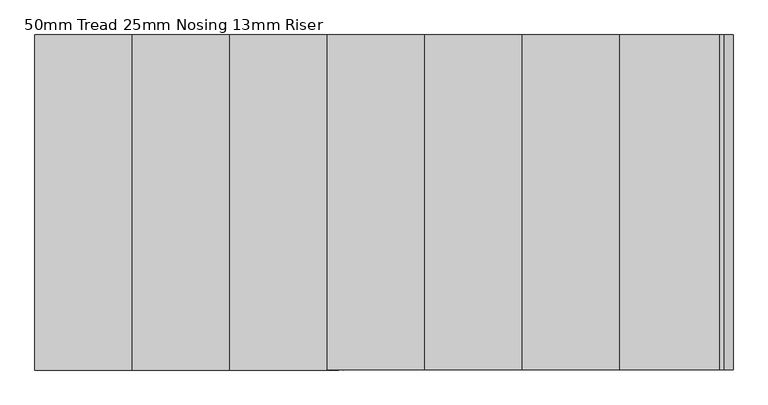
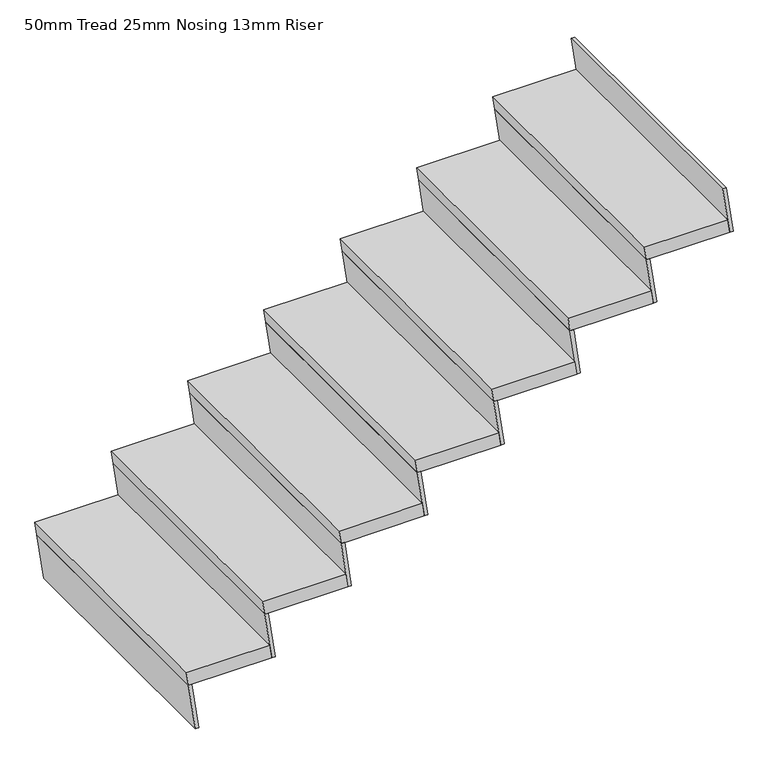
"""IFC4 building model written with IfcOpenShell, lengths in millimetres: stair flight geometry, 50mm Tread 25mm Nosing 13mm Riser."""

from ifc_helpers import new_model, si_unit, frame, origin, place, context, project, spatial, polyline, outline, extrude, source, transform, mapped, element, save


def stair_flight_50mm_tread_25mm_nosing_13mm_riser_6fe2c66d(model_context):
    return source(origin(), model_context, "Body", "SweptSolid", [
        extrude(outline(polyline([(1217.3913043, -932.4697153), (1217.3913043, -1232.4697153), (1167.3913043, -1225.2822153), (1167.3913043, -925.2822153), (1217.3913043, -932.4697153)])), frame((0.0, 1980.9593033, 0.0), z_axis=(0.0, 1.0, 0.0), x_axis=(0.0, 0.0, 1.0)), (0.0, 0.0, 1.0), 945.271643),
        extrude(outline(polyline([(1167.3913043, -1225.2822153), (993.4782609, -1200.2822153), (993.4782609, -1187.6537253), (1167.3913043, -1212.6537253), (1167.3913043, -1225.2822153)])), frame((0.0, 1980.9593033, 0.0), z_axis=(0.0, 1.0, 0.0), x_axis=(0.0, 0.0, 1.0)), (0.0, 0.0, 1.0), 945.271643),
        extrude(outline(polyline([(1341.3043478, -950.2822153), (1167.3913043, -925.2822153), (1167.3913043, -912.6537253), (1341.3043478, -937.6537253), (1341.3043478, -950.2822153)])), frame((0.0, 1980.9593033, 0.0), z_axis=(0.0, 1.0, 0.0), x_axis=(0.0, 0.0, 1.0)), (0.0, 0.0, 1.0), 945.271643),
        extrude(outline(polyline([(1391.3043478, -657.4697153), (1391.3043478, -957.4697153), (1341.3043478, -950.2822153), (1341.3043478, -650.2822153), (1391.3043478, -657.4697153)])), frame((0.0, 1980.9593033, 0.0), z_axis=(0.0, 1.0, 0.0), x_axis=(0.0, 0.0, 1.0)), (0.0, 0.0, 1.0), 945.271643),
        extrude(outline(polyline([(1515.2173913, -675.2822153), (1341.3043478, -650.2822153), (1341.3043478, -637.6537253), (1515.2173913, -662.6537253), (1515.2173913, -675.2822153)])), frame((0.0, 1980.9593033, 0.0), z_axis=(0.0, 1.0, 0.0), x_axis=(0.0, 0.0, 1.0)), (0.0, 0.0, 1.0), 945.271643),
        extrude(outline(polyline([(1565.2173913, -382.4697153), (1565.2173913, -682.4697153), (1515.2173913, -675.2822153), (1515.2173913, -375.2822153), (1565.2173913, -382.4697153)])), frame((0.0, 1980.9593033, 0.0), z_axis=(0.0, 1.0, 0.0), x_axis=(0.0, 0.0, 1.0)), (0.0, 0.0, 1.0), 945.271643),
        extrude(outline(polyline([(1689.1304348, -400.2822153), (1515.2173913, -375.2822153), (1515.2173913, -362.6537253), (1689.1304348, -387.6537253), (1689.1304348, -400.2822153)])), frame((0.0, 1980.9593033, 0.0), z_axis=(0.0, 1.0, 0.0), x_axis=(0.0, 0.0, 1.0)), (0.0, 0.0, 1.0), 945.271643),
        extrude(outline(polyline([(1739.1304348, -107.4697153), (1739.1304348, -407.4697153), (1689.1304348, -400.2822153), (1689.1304348, -100.2822153), (1739.1304348, -107.4697153)])), frame((0.0, 1980.9593033, 0.0), z_axis=(0.0, 1.0, 0.0), x_axis=(0.0, 0.0, 1.0)), (0.0, 0.0, 1.0), 945.271643),
        extrude(outline(polyline([(1863.0434783, -125.2822153), (1689.1304348, -100.2822153), (1689.1304348, -87.6537253), (1863.0434783, -112.6537253), (1863.0434783, -125.2822153)])), frame((0.0, 1980.9593033, 0.0), z_axis=(0.0, 1.0, 0.0), x_axis=(0.0, 0.0, 1.0)), (0.0, 0.0, 1.0), 945.271643),
        extrude(outline(polyline([(1913.0434783, 167.5302847), (1913.0434783, -132.4697153), (1863.0434783, -125.2822153), (1863.0434783, 174.7177847), (1913.0434783, 167.5302847)])), frame((0.0, 1980.9593033, 0.0), z_axis=(0.0, 1.0, 0.0), x_axis=(0.0, 0.0, 1.0)), (0.0, 0.0, 1.0), 945.271643),
        extrude(outline(polyline([(2036.9565217, 149.7177847), (1863.0434783, 174.7177847), (1863.0434783, 187.3462747), (2036.9565217, 162.3462747), (2036.9565217, 149.7177847)])), frame((0.0, 1980.9593033, 0.0), z_axis=(0.0, 1.0, 0.0), x_axis=(0.0, 0.0, 1.0)), (0.0, 0.0, 1.0), 945.271643),
        extrude(outline(polyline([(2086.9565217, 442.5302847), (2086.9565217, 142.5302847), (2036.9565217, 149.7177847), (2036.9565217, 449.7177847), (2086.9565217, 442.5302847)])), frame((0.0, 1980.9593033, 0.0), z_axis=(0.0, 1.0, 0.0), x_axis=(0.0, 0.0, 1.0)), (0.0, 0.0, 1.0), 945.271643),
        extrude(outline(polyline([(2210.8695652, 424.7177847), (2036.9565217, 449.7177847), (2036.9565217, 462.3462747), (2210.8695652, 437.3462747), (2210.8695652, 424.7177847)])), frame((0.0, 1980.9593033, 0.0), z_axis=(0.0, 1.0, 0.0), x_axis=(0.0, 0.0, 1.0)), (0.0, 0.0, 1.0), 945.271643),
        extrude(outline(polyline([(2384.7826087, 699.7177847), (2210.8695652, 724.7177847), (2210.8695652, 737.3462747), (2384.7826087, 712.3462747), (2384.7826087, 699.7177847)])), frame((0.0, 1980.9593033, 0.0), z_axis=(0.0, 1.0, 0.0), x_axis=(0.0, 0.0, 1.0)), (0.0, 0.0, 1.0), 945.271643),
        extrude(outline(polyline([(2260.8695652, 717.5302847), (2260.8695652, 417.5302847), (2210.8695652, 424.7177847), (2210.8695652, 724.7177847), (2260.8695652, 717.5302847)])), frame((0.0, 1980.9593033, 0.0), z_axis=(0.0, 1.0, 0.0), x_axis=(0.0, 0.0, 1.0)), (0.0, 0.0, 1.0), 945.271643),
    ])


if __name__ == "__main__":
    model = new_model("IFC4")
    model_context = context("Model", 3, world=origin())
    ifc_project = project(units=[si_unit("LENGTHUNIT", "METRE", prefix="MILLI")], contexts=[model_context])
    site = spatial("IfcSite", under=ifc_project)
    building = spatial("IfcBuilding", under=site)
    placement = place(None, origin())
    stair_flight_50mm_tread_25mm_nosing_13mm_riser_shape = stair_flight_50mm_tread_25mm_nosing_13mm_riser_6fe2c66d(model_context)
    element("IfcStairFlight", 1, ObjectType="50mm Tread 25mm Nosing 13mm Riser", at=placement, inside=building, context=model_context, shape_type="MappedRepresentation", body=[
        mapped(stair_flight_50mm_tread_25mm_nosing_13mm_riser_shape, transform((0.0, 0.0, 0.0), x_axis=(1.0, 0.0, 0.0), y_axis=(0.0, 1.0, 0.0), z_axis=(0.0, 0.0, 1.0))),
    ])
    save(model, "model.ifc")
